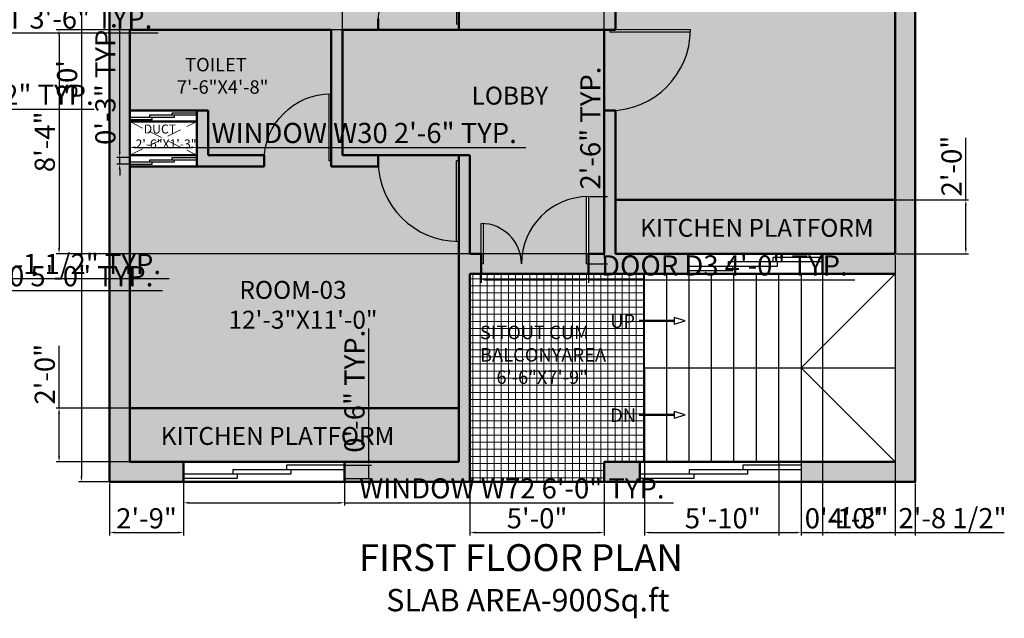
# Model space of a CAD drawing. Units: inches. Extents: x 3274 to 5176, y 1085 to 2172.
# Tile 9 of 16: x 3740 to 4180, y 1614 to 1881. Entities that reach past the tile are written whole.
import ezdxf

# ---------------------------------------------------------------- set-up
doc = ezdxf.new("R2010")
doc.units = ezdxf.units.IN
doc.linetypes.add('DASHED', pattern=[19.05, 12.7, -6.35])
for name, color, linetype, lineweight in [('A-ANNO-DIMS', 2, 'Continuous', 18), ('A-ANNO-TEXT', 7, 'Continuous', 25), ('A-AREA-IDEN', 3, 'Continuous', 25), ('A-DOOR', 4, 'Continuous', 25), ('A-FLOR-OPEN', 7, 'DASHED', 18), ('A-FLOR-PATT', 252, 'Continuous', 13), ('A-FLOR-STRS', 7, 'Continuous', 25), ('A-GLAZ', 5, 'Continuous', 25), ('A-WALL', 7, 'Continuous', 50), ('A-WALL-PATT', 8, 'Continuous', 13)]:
    doc.layers.add(name, color=color, linetype=linetype, lineweight=lineweight)
doc.styles.get("Standard").update_dxf_attribs({"font": 'arial.ttf'})
doc.dimstyles.new('ISO-25', dxfattribs={"dimtxt": 9, "dimasz": 2.5, "dimexe": 1.25, "dimexo": 0.625, "dimtad": 1, "dimdec": 1, "dimlunit": 3, "dimtxsty": 'Standard', "dimcen": 2.5, "dimclrd": 4, "dimclre": 4, "dimclrt": 1, "dimadec": 0, "dimazin": 0, "dimtfac": 1, "dimtdec": 1, "dimtmove": 0, "dimatfit": 3, "dimfxl": 1, "dimarcsym": 0})

# ---------------------------------------------------------------- blocks, each defined once
blk = doc.blocks.new('*D66')
at = {"layer": 'A-ANNO-DIMS', "color": 0, "lineweight": -2, "transparency": 16777216}
for p, q in [((3779.1, 2034.48), (3765.87, 2034.48)), ((3767.12, 2031.98), (3767.12, 1676.98)), ((3779.1, 1674.48), (3765.87, 1674.48))]:
    blk.add_line(p, q, dxfattribs=at)
at = {"layer": 'A-ANNO-DIMS', "color": 0, "transparency": 16777216}
for points in [[(3766.71, 2031.98), (3767.54, 2031.98), (3767.12, 2034.48)], [(3766.71, 1676.98), (3767.54, 1676.98), (3767.12, 1674.48)]]:
    blk.add_solid(points, dxfattribs=at)
at = {"layer": 'Defpoints', "color": 0, "transparency": 16777216}
for p in [(3779.73, 2034.48), (3767.12, 1674.48), (3779.73, 1674.48)]:
    blk.add_point(p, dxfattribs=at)
at = {"layer": 'A-ANNO-DIMS', "color": 0, "transparency": 16777216, "insert": (3761.9, 1854.48), "char_height": 9, "attachment_point": 5, "rotation": 90}
blk.add_mtext("30'", dxfattribs=at)
blk = doc.blocks.new('1')
for p, q in [((0, 36), (0, 0)), ((1, 36), (1, 0)), ((0, 0), (1, 0))]:
    blk.add_line(p, q)
blk.add_arc((0, 0), 36, 0, 90)
blk = doc.blocks.new('3')
for p, q in [((47, 30), (47, 0)), ((48, 30), (48, 0)), ((0, 0), (0, 18)), ((1, 0), (1, 18)), ((1, 0), (0, 0)), ((48, 0), (47, 0))]:
    blk.add_line(p, q)
for centre, radius, start, end in [((48, 0), 30, 90, 180), ((0, 0), 18, 0, 90)]:
    blk.add_arc(centre, radius, start, end)
blk = doc.blocks.new('2')
for p, q in [((0, 30), (0, 0)), ((1, 30), (1, 0)), ((0, 0), (1, 0))]:
    blk.add_line(p, q)
blk.add_arc((0, 0), 30, 0, 90)
blk = doc.blocks.new('WIN-30')
for p, q in [((4366.19, 1316.35), (4386.19, 1316.35)), ((4375.19, 1317.35), (4396.19, 1317.35)), ((4375.19, 1316.35), (4375.19, 1317.35)), ((4376.19, 1315.35), (4376.19, 1316.35)), ((4385.19, 1318.35), (4396.19, 1318.35)), ((4385.19, 1317.35), (4385.19, 1318.35)), ((4386.19, 1316.35), (4386.19, 1317.35)), ((4366.19, 1315.35), (4376.19, 1315.35))]:
    blk.add_line(p, q)
blk = doc.blocks.new('WIN-60')
for p, q in [((4598.19, 1271.85), (4640.19, 1271.85)), ((4598.19, 1269.85), (4598.19, 1271.85)), ((4618.19, 1273.85), (4640.19, 1273.85)), ((4618.19, 1271.85), (4618.19, 1273.85)), ((4620.19, 1269.85), (4620.19, 1271.85)), ((4580.19, 1269.85), (4620.19, 1269.85)), ((4580.19, 1267.85), (4600.19, 1267.85)), ((4600.19, 1267.85), (4600.19, 1269.85))]:
    blk.add_line(p, q)
blk = doc.blocks.new('WIN-72')
for p, q in [((4462.19, 1180.85), (4436.19, 1180.85)), ((4436.19, 1180.85), (4436.19, 1178.85)), ((4438.19, 1176.85), (4390.19, 1176.85)), ((4414.19, 1174.85), (4390.19, 1174.85)), ((4462.19, 1178.85), (4412.19, 1178.85)), ((4412.19, 1178.85), (4412.19, 1176.85)), ((4414.19, 1176.85), (4414.19, 1174.85)), ((4438.19, 1178.85), (4438.19, 1176.85))]:
    blk.add_line(p, q)
blk = doc.blocks.new('*D118')
at = {"layer": 'A-ANNO-DIMS', "color": 4, "lineweight": -2, "transparency": 16777216}
for p, q in [((3945.73, 1771.36), (3945.73, 1763.53)), ((3993.73, 1771.36), (3993.73, 1763.53)), ((3948.23, 1764.78), (3991.23, 1764.78)), ((3993.73, 1764.78), (4112.67, 1764.78))]:
    blk.add_line(p, q, dxfattribs=at)
at = {"layer": 'A-ANNO-DIMS', "color": 4, "transparency": 16777216}
for points in [[(3948.23, 1765.2), (3948.23, 1764.37), (3945.73, 1764.78)], [(3991.23, 1765.2), (3991.23, 1764.37), (3993.73, 1764.78)]]:
    blk.add_solid(points, dxfattribs=at)
at = {"layer": 'Defpoints', "color": 0, "transparency": 16777216}
for p in [(3945.73, 1771.98), (3993.73, 1771.98), (3993.73, 1764.78)]:
    blk.add_point(p, dxfattribs=at)
at = {"layer": 'A-ANNO-DIMS', "color": 1, "transparency": 16777216, "insert": (4054.45, 1770.07), "char_height": 9, "attachment_point": 5}
blk.add_mtext('DOOR D3 4\'-0" TYP.', dxfattribs=at)
blk = doc.blocks.new('*D119')
at = {"layer": 'A-ANNO-DIMS', "color": 4, "lineweight": -2, "transparency": 16777216}
for p, q in [((4000.93, 1801.98), (4000.93, 1860.75)), ((3994.35, 1801.98), (4002.18, 1801.98)), ((4000.93, 1774.48), (4000.93, 1799.48)), ((3994.35, 1771.98), (4002.18, 1771.98))]:
    blk.add_line(p, q, dxfattribs=at)
at = {"layer": 'A-ANNO-DIMS', "color": 4, "transparency": 16777216}
for points in [[(4000.51, 1799.48), (4001.35, 1799.48), (4000.93, 1801.98)], [(4000.51, 1774.48), (4001.35, 1774.48), (4000.93, 1771.98)]]:
    blk.add_solid(points, dxfattribs=at)
at = {"layer": 'Defpoints', "color": 0, "transparency": 16777216}
for p in [(3993.73, 1801.98), (4000.93, 1801.98), (3993.73, 1771.98)]:
    blk.add_point(p, dxfattribs=at)
at = {"layer": 'A-ANNO-DIMS', "color": 1, "transparency": 16777216, "insert": (3995.71, 1832.61), "char_height": 9, "attachment_point": 5, "rotation": 90}
blk.add_mtext('2\'-6" TYP.', dxfattribs=at)
blk = doc.blocks.new('*D120')
at = {"layer": 'A-ANNO-DIMS', "color": 4, "lineweight": -2, "transparency": 16777216}
for p, q in [((3788.73, 1820.11), (3788.73, 1825.23)), ((3791.23, 1823.98), (3816.23, 1823.98)), ((3818.73, 1820.11), (3818.73, 1825.23)), ((3818.73, 1823.98), (3965.71, 1823.98))]:
    blk.add_line(p, q, dxfattribs=at)
at = {"layer": 'A-ANNO-DIMS', "color": 4, "transparency": 16777216}
for points in [[(3791.23, 1824.4), (3791.23, 1823.57), (3788.73, 1823.98)], [(3816.23, 1824.4), (3816.23, 1823.57), (3818.73, 1823.98)]]:
    blk.add_solid(points, dxfattribs=at)
at = {"layer": 'Defpoints', "color": 0, "transparency": 16777216}
for p in [(3818.73, 1823.98), (3788.73, 1819.48), (3818.73, 1819.48)]:
    blk.add_point(p, dxfattribs=at)
at = {"layer": 'A-ANNO-DIMS', "color": 1, "transparency": 16777216, "insert": (3893.47, 1829.27), "char_height": 9, "attachment_point": 5}
blk.add_mtext('WINDOW W30 2\'-6" TYP.', dxfattribs=at)
blk = doc.blocks.new('*D121')
at = {"layer": 'A-ANNO-DIMS', "color": 4, "lineweight": -2, "transparency": 16777216}
for p, q in [((3784.23, 1821.98), (3784.23, 1880.59)), ((3788.1, 1819.48), (3782.98, 1819.48)), ((3784.23, 1816.48), (3784.23, 1819.48)), ((3788.1, 1816.48), (3782.98, 1816.48)), ((3784.23, 1813.98), (3784.23, 1811.48))]:
    blk.add_line(p, q, dxfattribs=at)
at = {"layer": 'A-ANNO-DIMS', "color": 4, "transparency": 16777216}
for points in [[(3783.81, 1821.98), (3784.65, 1821.98), (3784.23, 1819.48)], [(3783.81, 1813.98), (3784.65, 1813.98), (3784.23, 1816.48)]]:
    blk.add_solid(points, dxfattribs=at)
at = {"layer": 'Defpoints', "color": 0, "transparency": 16777216}
for p in [(3784.23, 1819.48), (3788.73, 1819.48), (3788.73, 1816.48)]:
    blk.add_point(p, dxfattribs=at)
at = {"layer": 'A-ANNO-DIMS', "color": 1, "transparency": 16777216, "insert": (3779.01, 1852.54), "char_height": 9, "attachment_point": 5, "rotation": 90}
blk.add_mtext('0\'-3" TYP.', dxfattribs=at)
blk = doc.blocks.new('*D124')
at = {"layer": 'A-ANNO-DIMS', "color": 4, "lineweight": -2, "transparency": 16777216}
for p, q in [((3812.73, 1675.36), (3812.73, 1663.93)), ((3884.73, 1675.36), (3884.73, 1663.93)), ((3815.23, 1665.18), (3882.23, 1665.18)), ((3884.73, 1665.18), (4031.71, 1665.18))]:
    blk.add_line(p, q, dxfattribs=at)
at = {"layer": 'A-ANNO-DIMS', "color": 4, "transparency": 16777216}
for points in [[(3815.23, 1665.6), (3815.23, 1664.77), (3812.73, 1665.18)], [(3882.23, 1665.6), (3882.23, 1664.77), (3884.73, 1665.18)]]:
    blk.add_solid(points, dxfattribs=at)
at = {"layer": 'Defpoints', "color": 0, "transparency": 16777216}
for p in [(3812.73, 1675.98), (3884.73, 1675.98), (3884.73, 1665.18)]:
    blk.add_point(p, dxfattribs=at)
at = {"layer": 'A-ANNO-DIMS', "color": 1, "transparency": 16777216, "insert": (3959.47, 1670.46), "char_height": 9, "attachment_point": 5}
blk.add_mtext('WINDOW W72 6\'-0" TYP.', dxfattribs=at)
blk = doc.blocks.new('*D125')
at = {"layer": 'A-ANNO-DIMS', "color": 4, "lineweight": -2, "transparency": 16777216}
for p, q in [((3895.53, 1684.48), (3895.53, 1743.09)), ((3885.35, 1681.98), (3896.78, 1681.98)), ((3895.53, 1675.98), (3895.53, 1681.98)), ((3885.35, 1675.98), (3896.78, 1675.98)), ((3895.53, 1673.48), (3895.53, 1670.98))]:
    blk.add_line(p, q, dxfattribs=at)
at = {"layer": 'A-ANNO-DIMS', "color": 4, "transparency": 16777216}
for points in [[(3895.11, 1684.48), (3895.95, 1684.48), (3895.53, 1681.98)], [(3895.11, 1673.48), (3895.95, 1673.48), (3895.53, 1675.98)]]:
    blk.add_solid(points, dxfattribs=at)
at = {"layer": 'Defpoints', "color": 0, "transparency": 16777216}
for p in [(3884.73, 1681.98), (3895.53, 1681.98), (3884.73, 1675.98)]:
    blk.add_point(p, dxfattribs=at)
at = {"layer": 'A-ANNO-DIMS', "color": 1, "transparency": 16777216, "insert": (3890.31, 1715.04), "char_height": 9, "attachment_point": 5, "rotation": 90}
blk.add_mtext('0\'-6" TYP.', dxfattribs=at)
blk = doc.blocks.new('*D128')
at = {"layer": 'A-ANNO-DIMS', "color": 4, "lineweight": -2, "transparency": 16777216}
for p, q in [((3596.3, 1768.36), (3596.3, 1758.73)), ((3656.3, 1768.36), (3656.3, 1758.73)), ((3598.8, 1759.98), (3653.8, 1759.98)), ((3656.3, 1759.98), (3803.28, 1759.98))]:
    blk.add_line(p, q, dxfattribs=at)
at = {"layer": 'A-ANNO-DIMS', "color": 4, "transparency": 16777216}
for points in [[(3598.8, 1760.4), (3598.8, 1759.57), (3596.3, 1759.98)], [(3653.8, 1760.4), (3653.8, 1759.57), (3656.3, 1759.98)]]:
    blk.add_solid(points, dxfattribs=at)
at = {"layer": 'Defpoints', "color": 0, "transparency": 16777216}
for p in [(3596.3, 1768.98), (3656.3, 1768.98), (3656.3, 1759.98)]:
    blk.add_point(p, dxfattribs=at)
at = {"layer": 'A-ANNO-DIMS', "color": 1, "transparency": 16777216, "insert": (3731.04, 1765.26), "char_height": 9, "attachment_point": 5}
blk.add_mtext('WINDOW W60 5\'-0" TYP.', dxfattribs=at)
blk = doc.blocks.new('*D130')
at = {"layer": 'A-ANNO-DIMS', "color": 4, "lineweight": -2, "transparency": 16777216}
for p, q in [((3648.04, 1880.86), (3648.04, 1873.91)), ((3690.17, 1880.86), (3690.17, 1873.91)), ((3650.54, 1875.16), (3687.67, 1875.16)), ((3690.17, 1875.16), (3801.39, 1875.16))]:
    blk.add_line(p, q, dxfattribs=at)
at = {"layer": 'A-ANNO-DIMS', "color": 4, "transparency": 16777216}
for points in [[(3650.54, 1875.58), (3650.54, 1874.75), (3648.04, 1875.16)], [(3687.67, 1875.58), (3687.67, 1874.75), (3690.17, 1875.16)]]:
    blk.add_solid(points, dxfattribs=at)
at = {"layer": 'Defpoints', "color": 0, "transparency": 16777216}
for p in [(3648.04, 1881.48), (3690.17, 1881.48), (3690.17, 1875.16)]:
    blk.add_point(p, dxfattribs=at)
at = {"layer": 'A-ANNO-DIMS', "color": 1, "transparency": 16777216, "insert": (3747.03, 1880.39), "char_height": 9, "attachment_point": 5}
blk.add_mtext('TV UNIT 3\'-6" TYP.', dxfattribs=at)
blk = doc.blocks.new('*D139')
at = {"layer": 'A-ANNO-DIMS', "color": 4, "lineweight": -2, "transparency": 16777216}
for p, q in [((3664.71, 1838.01), (3664.71, 1842.31)), ((3667.21, 1841.06), (3684.52, 1841.06)), ((3687.02, 1838.01), (3687.02, 1842.31)), ((3687.02, 1841.06), (3772.75, 1841.06))]:
    blk.add_line(p, q, dxfattribs=at)
at = {"layer": 'A-ANNO-DIMS', "color": 4, "transparency": 16777216}
for points in [[(3667.21, 1841.48), (3667.21, 1840.65), (3664.71, 1841.06)], [(3684.52, 1841.48), (3684.52, 1840.65), (3687.02, 1841.06)]]:
    blk.add_solid(points, dxfattribs=at)
at = {"layer": 'Defpoints', "color": 0, "transparency": 16777216}
for p in [(3687.02, 1841.06), (3664.71, 1837.38), (3687.02, 1837.38)]:
    blk.add_point(p, dxfattribs=at)
at = {"layer": 'A-ANNO-DIMS', "color": 1, "transparency": 16777216, "insert": (3731.13, 1846.34), "char_height": 9, "attachment_point": 5}
blk.add_mtext('1\'-10 1/2" TYP.', dxfattribs=at)
blk = doc.blocks.new('*D140')
at = {"layer": 'A-ANNO-DIMS', "color": 4, "lineweight": -2, "transparency": 16777216}
for p, q in [((3596.75, 1775.85), (3596.75, 1764.21)), ((3670.16, 1775.85), (3670.16, 1764.21)), ((3599.25, 1765.46), (3667.66, 1765.46)), ((3670.16, 1765.46), (3806.3, 1765.46))]:
    blk.add_line(p, q, dxfattribs=at)
at = {"layer": 'A-ANNO-DIMS', "color": 4, "transparency": 16777216}
for points in [[(3599.25, 1765.88), (3599.25, 1765.04), (3596.75, 1765.46)], [(3667.66, 1765.88), (3667.66, 1765.04), (3670.16, 1765.46)]]:
    blk.add_solid(points, dxfattribs=at)
at = {"layer": 'Defpoints', "color": 0, "transparency": 16777216}
for p in [(3596.75, 1776.47), (3670.16, 1776.47), (3670.16, 1765.46)]:
    blk.add_point(p, dxfattribs=at)
at = {"layer": 'A-ANNO-DIMS', "color": 1, "transparency": 16777216, "insert": (3739.48, 1770.74), "char_height": 9, "attachment_point": 5}
blk.add_mtext('SOFA S1 6\'-1 1/2" TYP.', dxfattribs=at)
blk = doc.blocks.new('*D204')
at = {"layer": 'A-ANNO-DIMS', "color": 4, "lineweight": -2, "transparency": 16777216}
for p, q in [((3779.73, 1673.86), (3779.73, 1650.63)), ((3812.73, 1673.86), (3812.73, 1650.63)), ((3782.23, 1651.88), (3810.23, 1651.88))]:
    blk.add_line(p, q, dxfattribs=at)
at = {"layer": 'A-ANNO-DIMS', "color": 4, "transparency": 16777216}
for points in [[(3782.23, 1652.3), (3782.23, 1651.47), (3779.73, 1651.88)], [(3810.23, 1652.3), (3810.23, 1651.47), (3812.73, 1651.88)]]:
    blk.add_solid(points, dxfattribs=at)
at = {"layer": 'Defpoints', "color": 0, "transparency": 16777216}
for p in [(3779.73, 1674.48), (3812.73, 1674.48), (3812.73, 1651.88)]:
    blk.add_point(p, dxfattribs=at)
at = {"layer": 'A-ANNO-DIMS', "color": 1, "transparency": 16777216, "insert": (3796.23, 1657.1), "char_height": 9, "attachment_point": 5}
blk.add_mtext('2\'-9"', dxfattribs=at)
blk = doc.blocks.new('*D205')
at = {"layer": 'A-ANNO-DIMS', "color": 4, "lineweight": -2, "transparency": 16777216}
for p, q in [((4088.73, 1673.86), (4088.73, 1650.63)), ((4139.73, 1673.86), (4139.73, 1650.63)), ((4091.23, 1651.88), (4137.23, 1651.88))]:
    blk.add_line(p, q, dxfattribs=at)
at = {"layer": 'A-ANNO-DIMS', "color": 4, "transparency": 16777216}
for points in [[(4091.23, 1652.3), (4091.23, 1651.47), (4088.73, 1651.88)], [(4137.23, 1652.3), (4137.23, 1651.47), (4139.73, 1651.88)]]:
    blk.add_solid(points, dxfattribs=at)
at = {"layer": 'Defpoints', "color": 0, "transparency": 16777216}
for p in [(4088.73, 1674.48), (4139.73, 1674.48), (4139.73, 1651.88)]:
    blk.add_point(p, dxfattribs=at)
at = {"layer": 'A-ANNO-DIMS', "color": 1, "transparency": 16777216, "insert": (4114.23, 1657.11), "char_height": 9, "attachment_point": 5}
blk.add_mtext('4\'-3"', dxfattribs=at)
blk = doc.blocks.new('*D206')
at = {"layer": 'A-ANNO-DIMS', "color": 4, "lineweight": -2, "transparency": 16777216}
for p, q in [((3940.73, 1673.86), (3940.73, 1650.63)), ((4000.73, 1673.86), (4000.73, 1650.63)), ((3943.23, 1651.88), (3998.23, 1651.88))]:
    blk.add_line(p, q, dxfattribs=at)
at = {"layer": 'A-ANNO-DIMS', "color": 4, "transparency": 16777216}
for points in [[(3943.23, 1652.3), (3943.23, 1651.47), (3940.73, 1651.88)], [(3998.23, 1652.3), (3998.23, 1651.47), (4000.73, 1651.88)]]:
    blk.add_solid(points, dxfattribs=at)
at = {"layer": 'Defpoints', "color": 0, "transparency": 16777216}
for p in [(3940.73, 1674.48), (4000.73, 1674.48), (4000.73, 1651.88)]:
    blk.add_point(p, dxfattribs=at)
at = {"layer": 'A-ANNO-DIMS', "color": 1, "transparency": 16777216, "insert": (3970.73, 1657.1), "char_height": 9, "attachment_point": 5}
blk.add_mtext('5\'-0"', dxfattribs=at)
blk = doc.blocks.new('*D207')
at = {"layer": 'A-ANNO-DIMS', "color": 4, "lineweight": -2, "transparency": 16777216}
for p, q in [((3757.13, 1707.48), (3757.13, 1735.31)), ((3935.1, 1707.48), (3755.88, 1707.48)), ((3757.13, 1685.98), (3757.13, 1704.98)), ((3935.1, 1683.48), (3755.88, 1683.48))]:
    blk.add_line(p, q, dxfattribs=at)
at = {"layer": 'A-ANNO-DIMS', "color": 4, "transparency": 16777216}
for points in [[(3756.71, 1704.98), (3757.55, 1704.98), (3757.13, 1707.48)], [(3756.71, 1685.98), (3757.55, 1685.98), (3757.13, 1683.48)]]:
    blk.add_solid(points, dxfattribs=at)
at = {"layer": 'Defpoints', "color": 0, "transparency": 16777216}
for p in [(3757.13, 1707.48), (3935.73, 1707.48), (3935.73, 1683.48)]:
    blk.add_point(p, dxfattribs=at)
at = {"layer": 'A-ANNO-DIMS', "color": 1, "transparency": 16777216, "insert": (3751.91, 1722.65), "char_height": 9, "attachment_point": 5, "rotation": 90}
blk.add_mtext('2\'-0"', dxfattribs=at)
blk = doc.blocks.new('*D209')
at = {"layer": 'A-ANNO-DIMS', "color": 4, "lineweight": -2, "transparency": 16777216}
for p, q in [((4162.33, 1800.48), (4162.33, 1828.31)), ((4131.35, 1800.48), (4163.58, 1800.48)), ((4162.33, 1778.98), (4162.33, 1797.98)), ((4131.35, 1776.48), (4163.58, 1776.48))]:
    blk.add_line(p, q, dxfattribs=at)
at = {"layer": 'A-ANNO-DIMS', "color": 4, "transparency": 16777216}
for points in [[(4161.91, 1797.98), (4162.75, 1797.98), (4162.33, 1800.48)], [(4161.91, 1778.98), (4162.75, 1778.98), (4162.33, 1776.48)]]:
    blk.add_solid(points, dxfattribs=at)
at = {"layer": 'Defpoints', "color": 0, "transparency": 16777216}
for p in [(4130.73, 1800.48), (4162.33, 1800.48), (4130.73, 1776.48)]:
    blk.add_point(p, dxfattribs=at)
at = {"layer": 'A-ANNO-DIMS', "color": 1, "transparency": 16777216, "insert": (4157.11, 1815.65), "char_height": 9, "attachment_point": 5, "rotation": 90}
blk.add_mtext('2\'-0"', dxfattribs=at)
blk = doc.blocks.new('*D210')
at = {"layer": 'A-ANNO-DIMS', "color": 4, "lineweight": -2, "transparency": 16777216}
for p, q in [((4018.73, 1724.86), (4018.73, 1650.63)), ((4088.73, 1724.86), (4088.73, 1650.63)), ((4021.23, 1651.88), (4086.23, 1651.88))]:
    blk.add_line(p, q, dxfattribs=at)
at = {"layer": 'A-ANNO-DIMS', "color": 4, "transparency": 16777216}
for points in [[(4021.23, 1652.3), (4021.23, 1651.47), (4018.73, 1651.88)], [(4086.23, 1652.3), (4086.23, 1651.47), (4088.73, 1651.88)]]:
    blk.add_solid(points, dxfattribs=at)
at = {"layer": 'Defpoints', "color": 0, "transparency": 16777216}
for p in [(4018.73, 1725.48), (4088.73, 1725.48), (4088.73, 1651.88)]:
    blk.add_point(p, dxfattribs=at)
at = {"layer": 'A-ANNO-DIMS', "color": 1, "transparency": 16777216, "insert": (4053.73, 1657.1), "char_height": 9, "attachment_point": 5}
blk.add_mtext('5\'-10"', dxfattribs=at)
blk = doc.blocks.new('*D211')
at = {"layer": 'A-ANNO-DIMS', "color": 4, "lineweight": -2, "transparency": 16777216}
for p, q in [((4078.73, 1682.86), (4078.73, 1650.63)), ((4088.73, 1682.86), (4088.73, 1650.63)), ((4081.23, 1651.88), (4086.23, 1651.88)), ((4088.73, 1651.88), (4123.4, 1651.88))]:
    blk.add_line(p, q, dxfattribs=at)
at = {"layer": 'A-ANNO-DIMS', "color": 4, "transparency": 16777216}
for points in [[(4081.23, 1652.3), (4081.23, 1651.47), (4078.73, 1651.88)], [(4086.23, 1652.3), (4086.23, 1651.47), (4088.73, 1651.88)]]:
    blk.add_solid(points, dxfattribs=at)
at = {"layer": 'Defpoints', "color": 0, "transparency": 16777216}
for p in [(4078.73, 1683.48), (4088.73, 1683.48), (4088.73, 1651.88)]:
    blk.add_point(p, dxfattribs=at)
at = {"layer": 'A-ANNO-DIMS', "color": 1, "transparency": 16777216, "insert": (4107.31, 1657.1), "char_height": 9, "attachment_point": 5}
blk.add_mtext('0\'-10"', dxfattribs=at)
blk = doc.blocks.new('*D212')
at = {"layer": 'A-ANNO-DIMS', "color": 4, "lineweight": -2, "transparency": 16777216}
for p, q in [((3883.73, 1877.11), (3883.73, 2058.33)), ((3886.23, 2057.08), (3998.23, 2057.08)), ((4000.73, 1841.11), (4000.73, 2058.33))]:
    blk.add_line(p, q, dxfattribs=at)
at = {"layer": 'A-ANNO-DIMS', "color": 4, "transparency": 16777216}
for points in [[(3886.23, 2057.5), (3886.23, 2056.67), (3883.73, 2057.08)], [(3998.23, 2057.5), (3998.23, 2056.67), (4000.73, 2057.08)]]:
    blk.add_solid(points, dxfattribs=at)
at = {"layer": 'Defpoints', "color": 0, "transparency": 16777216}
for p in [(4000.73, 2057.08), (3883.73, 1876.48), (4000.73, 1840.48)]:
    blk.add_point(p, dxfattribs=at)
at = {"layer": 'A-ANNO-DIMS', "color": 1, "transparency": 16777216, "insert": (3942.23, 2062.3), "char_height": 9, "attachment_point": 5}
blk.add_mtext('9\'-9"', dxfattribs=at)
blk = doc.blocks.new('*D213')
at = {"layer": 'A-ANNO-DIMS', "color": 4, "lineweight": -2, "transparency": 16777216}
for p, q in [((3935.1, 1876.48), (3755.88, 1876.48)), ((3757.13, 1873.98), (3757.13, 1778.98)), ((4000.1, 1776.48), (3755.88, 1776.48))]:
    blk.add_line(p, q, dxfattribs=at)
at = {"layer": 'A-ANNO-DIMS', "color": 4, "transparency": 16777216}
for points in [[(3756.71, 1873.98), (3757.55, 1873.98), (3757.13, 1876.48)], [(3756.71, 1778.98), (3757.55, 1778.98), (3757.13, 1776.48)]]:
    blk.add_solid(points, dxfattribs=at)
at = {"layer": 'Defpoints', "color": 0, "transparency": 16777216}
for p in [(3935.73, 1876.48), (3757.13, 1776.48), (4000.73, 1776.48)]:
    blk.add_point(p, dxfattribs=at)
at = {"layer": 'A-ANNO-DIMS', "color": 1, "transparency": 16777216, "insert": (3751.91, 1826.48), "char_height": 9, "attachment_point": 5, "rotation": 90}
blk.add_mtext('8\'-4"', dxfattribs=at)
blk = doc.blocks.new('*D214')
at = {"layer": 'A-ANNO-DIMS', "color": 4, "lineweight": -2, "transparency": 16777216}
for p, q in [((4098.23, 1775.86), (4098.23, 1650.63)), ((4130.73, 1775.86), (4130.73, 1650.63)), ((4100.73, 1651.88), (4128.23, 1651.88)), ((4130.73, 1651.88), (4179.53, 1651.88))]:
    blk.add_line(p, q, dxfattribs=at)
at = {"layer": 'A-ANNO-DIMS', "color": 4, "transparency": 16777216}
for points in [[(4100.73, 1652.3), (4100.73, 1651.47), (4098.23, 1651.88)], [(4128.23, 1652.3), (4128.23, 1651.47), (4130.73, 1651.88)]]:
    blk.add_solid(points, dxfattribs=at)
at = {"layer": 'Defpoints', "color": 0, "transparency": 16777216}
for p in [(4098.23, 1776.48), (4130.73, 1776.48), (4130.73, 1651.88)]:
    blk.add_point(p, dxfattribs=at)
at = {"layer": 'A-ANNO-DIMS', "color": 1, "transparency": 16777216, "insert": (4156.38, 1657.16), "char_height": 9, "attachment_point": 5}
blk.add_mtext('2\'-8 1/2"', dxfattribs=at)

msp = doc.modelspace()

# ---------------------------------------------------------------- hatches: boundary and pattern name
at = {"layer": 'A-FLOR-PATT'}
h = msp.add_hatch(color=256, dxfattribs=at)
h.dxf.hatch_style = 1
h.paths.add_polyline_path([(4130.73, 2007.48), (4094.73, 2007.48), (4094.73, 1995.48), (4092.23, 1995.48, 0.404482), (4062.25, 1966.48), (4092.23, 1966.48), (4092.23, 1965.48), (4094.73, 1965.48), (4094.73, 1960.48), (4005.73, 1960.48), (4005.73, 1876.48), (4039.23, 1876.48, -0.394001), (4005.73, 1840.57), (4005.73, 1800.48), (4130.73, 1800.48)])
h.paths.add_polyline_path([(4089.73, 1995.38), (4089.73, 2025.48), (4005.73, 2025.48), (4005.73, 1965.48), (4062.23, 1965.48, -0.389983)])
h.paths.add_polyline_path([(4039.22, 1875.48), (4003.23, 1875.48), (4003.23, 1876.48), (4000.73, 1876.48), (4000.73, 1840.48), (4003.23, 1840.48, 0.4061)])
h.paths.add_polyline_path([(4043.84, 1879.07), (4112.24, 1879.07), (4112.24, 1908.93), (4043.84, 1908.93)], flags=24)
h.paths.add_polyline_path([(4026.66, 1988.49), (4068.63, 1988.49), (4068.63, 2010.88), (4026.66, 2010.88)], flags=24)
h = msp.add_hatch(color=256, dxfattribs=at)
h.dxf.hatch_style = 1
h.paths.add_polyline_path([(3938.23, 1949.48), (3935.73, 1949.48), (3935.73, 2001.48), (3788.73, 2001.48), (3788.73, 1881.48), (3899.82, 1881.48, -0.394001), (3935.73, 1914.98), (3935.73, 1919.48), (3938.23, 1919.48), (3938.23, 1920.48), (3968.21, 1920.48, 0.404482)])
h.paths.add_polyline_path([(3934.73, 1914.97, 0.4061), (3899.73, 1878.98), (3899.73, 1876.48), (3935.73, 1876.48), (3935.73, 1878.98), (3934.73, 1878.98)])
h.paths.add_polyline_path([(4000.73, 1984.48), (3940.73, 1984.48), (3940.73, 1949.38, -0.389983), (3968.23, 1919.48), (3940.73, 1919.48), (3940.73, 1881.48), (4000.73, 1881.48)])
h.paths.add_polyline_path([(3829.62, 1944.89), (3898.01, 1944.89), (3898.01, 1974.74), (3829.62, 1974.74)], flags=24)
h.paths.add_polyline_path([(3951.89, 1951.36), (3993.86, 1951.36), (3993.86, 1973.74), (3951.89, 1973.74)], flags=24)
h = msp.add_hatch(color=256, dxfattribs=at)
h.dxf.hatch_style = 1
h.paths.add_polyline_path([(3899.82, 1815.48), (3878.73, 1815.48), (3878.73, 1817.98), (3877.73, 1817.98), (3877.73, 1847.97, 0.404482), (3848.73, 1817.98), (3848.73, 1815.48), (3788.73, 1815.48), (3788.73, 1707.48), (3935.73, 1707.48), (3935.73, 1781.98, -0.394001)])
h.paths.add_polyline_path([(3878.73, 1847.98), (3878.73, 1876.48), (3788.73, 1876.48), (3788.73, 1840.48), (3823.73, 1840.48), (3823.73, 1820.48), (3848.83, 1820.48, -0.389983)])
h.paths.add_polyline_path([(3934.73, 1817.98), (3935.73, 1817.98), (3935.73, 1820.48), (3899.73, 1820.48), (3899.73, 1817.98, 0.4061), (3934.73, 1782)], flags=17)
h.paths.add_polyline_path([(3829.62, 1738.43), (3898.01, 1738.43), (3898.01, 1768.28), (3829.62, 1768.28)], flags=24)
h.paths.add_polyline_path([(3807.9, 1844.56), (3849.87, 1844.56), (3849.87, 1866.94), (3807.9, 1866.94)], flags=24)
h = msp.add_hatch(color=256, dxfattribs=at)
h.dxf.hatch_style = 1
h.paths.add_polyline_path([(3899.73, 1876.48), (3883.73, 1876.48), (3883.73, 1820.48), (3899.73, 1820.48), (3935.73, 1820.48), (3940.73, 1820.48), (3940.73, 1776.48), (3945.73, 1776.48), (3945.73, 1789.98, -0.414214), (3963.73, 1771.98, -0.404482), (3992.73, 1801.97), (3992.73, 1801.98), (3993.73, 1801.98), (3993.73, 1776.48), (4000.73, 1776.48), (4000.73, 1840.48), (4000.73, 1876.48), (3935.73, 1876.48)])
h.paths.add_polyline_path([(3963.73, 1771.98, 0.398025), (3946.73, 1789.96), (3946.73, 1771.98), (3945.73, 1767.48), (3993.73, 1767.48), (3993.73, 1771.98), (3992.73, 1771.98), (3992.73, 1801.97, 0.404482)])
h.paths.add_polyline_path([(3938.66, 1838.59), (3979.93, 1838.59), (3979.93, 1855.08), (3938.66, 1855.08)], flags=24)
h = msp.add_hatch(color=256, dxfattribs=at)
h.dxf.hatch_style = 1
h.paths.add_polyline_path([(4005.73, 1776.48), (4130.73, 1776.48), (4130.73, 1800.48), (4005.73, 1800.48)])
h.paths.add_polyline_path([(4013.96, 1779.54), (4130.97, 1779.54), (4130.97, 1796.03), (4013.96, 1796.03)], flags=9)
h = msp.add_hatch(dxfattribs=at)
h.set_pattern_fill('ANSI37', color=256, angle=45)
h.set_pattern_definition([(90, (-433.0866, 0), (-3.175, 0), []), (180, (-433.0866, 0), (-2e-16, -3.175), [])])
h.paths.add_polyline_path([(3940.73, 1674.48), (4000.73, 1674.48), (4000.73, 1683.48), (4018.73, 1683.48), (4018.73, 1725.48), (4018.73, 1767.48), (3993.73, 1767.48), (3945.73, 1767.48), (3940.73, 1767.48)])
h.paths.add_polyline_path([(3943.12, 1714.79), (4009.02, 1714.79), (4009.02, 1747.29), (3943.12, 1747.29)], flags=24)
h.paths.add_polyline_path([(4001.92, 1741.7), (4016.61, 1741.7), (4016.61, 1750.85), (4001.92, 1750.85)], flags=24)
h.paths.add_polyline_path([(4001.94, 1699.83), (4017.05, 1699.83), (4017.05, 1708.83), (4001.94, 1708.83)], flags=24)
h = msp.add_hatch(color=256, dxfattribs=at)
h.dxf.hatch_style = 1
h.paths.add_polyline_path([(3788.73, 1707.48), (3788.73, 1683.48), (3935.73, 1683.48), (3935.73, 1707.48)])
h.paths.add_polyline_path([(3799.76, 1686.54), (3916.77, 1686.54), (3916.77, 1703.03), (3799.76, 1703.03)], flags=24)
at = {"layer": 'A-WALL-PATT'}
h = msp.add_hatch(color=256, dxfattribs=at)
h.dxf.hatch_style = 1
h.paths.add_polyline_path([(3848.73, 1820.48), (3823.73, 1820.48), (3823.73, 1840.48), (3818.73, 1840.48), (3818.73, 1815.48), (3848.73, 1815.48)], flags=17)
h.paths.add_polyline_path([(3788.73, 1876.48), (3878.73, 1876.48), (3878.73, 1815.48), (3899.73, 1815.48), (3899.73, 1820.48), (3883.73, 1820.48), (3883.73, 1876.48), (3899.73, 1876.48), (3899.73, 1881.48), (3788.73, 1881.48), (3788.73, 2025.48), (4089.73, 2025.48), (4089.73, 1995.48), (4094.73, 1995.48), (4094.73, 2025.48), (4130.73, 2025.48), (4130.73, 1776.48), (4098.23, 1776.48), (4098.23, 1767.48), (4130.73, 1767.48), (4130.73, 1683.48), (4088.73, 1683.48), (4088.73, 1674.48), (4139.73, 1674.48), (4139.73, 2034.48), (3779.73, 2034.48), (3779.73, 1674.48), (3812.73, 1674.48), (3812.73, 1683.48), (3788.73, 1683.48)])
h.paths.add_polyline_path([(4005.73, 1989.48), (3982.73, 1989.48), (3982.73, 1984.48), (4000.73, 1984.48), (4000.73, 1881.48), (3940.73, 1881.48), (3940.73, 1919.48), (3938.23, 1919.48), (3935.73, 1919.48), (3935.73, 1876.48), (4005.73, 1876.48), (4005.73, 1960.48), (4094.73, 1960.48), (4094.73, 1965.48), (4005.73, 1965.48)], flags=17)
h.paths.add_polyline_path([(3958.73, 1989.48), (3935.73, 1989.48), (3935.73, 1949.48), (3940.73, 1949.48), (3940.73, 1984.48), (3958.73, 1984.48)], flags=17)
h.paths.add_polyline_path([(4038.23, 1776.48), (4005.73, 1776.48), (4005.73, 1840.48), (4000.73, 1840.48), (4000.73, 1776.48), (3993.73, 1776.48), (3993.73, 1771.98), (3993.73, 1767.48), (4038.23, 1767.48)], flags=17)
h.paths.add_polyline_path([(3940.73, 1767.48), (3945.73, 1767.48), (3945.73, 1776.48), (3940.73, 1776.48), (3940.73, 1820.48), (3935.73, 1820.48), (3935.73, 1683.48), (3884.73, 1683.48), (3884.73, 1674.48), (3940.73, 1674.48)], flags=17)
h.paths.add_polyline_path([(4016.73, 1683.48), (4000.73, 1683.48), (4000.73, 1674.48), (4016.73, 1674.48)], flags=17)

# ---------------------------------------------------------------- linework, layer by layer
at = {"layer": 'A-FLOR-OPEN', "ltscale": 0.5}
for p, q in [((3788.73, 1835.48), (3818.73, 1820.48)), ((3788.73, 1820.48), (3818.73, 1835.48))]:
    msp.add_line(p, q, dxfattribs=at)
at = {"layer": 'A-FLOR-STRS'}
for p, q in [((4018.73, 1725.48), (4018.73, 1767.48)), ((4028.73, 1725.48), (4028.73, 1767.48)), ((4038.73, 1725.48), (4038.73, 1767.48)), ((4048.73, 1725.48), (4048.73, 1767.48)), ((4058.73, 1725.48), (4058.73, 1767.48)), ((4068.73, 1725.48), (4068.73, 1767.48)), ((4078.73, 1725.48), (4078.73, 1767.48)), ((4088.73, 1767.48), (4088.73, 1683.48)), ((4088.73, 1725.48), (4130.73, 1767.48)), ((4130.73, 1767.48), (4130.73, 1683.48)), ((4018.73, 1725.48), (4130.73, 1725.48)), ((4018.73, 1683.48), (4018.73, 1725.48)), ((4028.73, 1683.48), (4028.73, 1725.48)), ((4038.73, 1683.48), (4038.73, 1725.48)), ((4048.73, 1683.48), (4048.73, 1725.48)), ((4058.73, 1683.48), (4058.73, 1725.48)), ((4068.73, 1683.48), (4068.73, 1725.48)), ((4078.73, 1683.48), (4078.73, 1725.48)), ((4088.73, 1725.48), (4130.73, 1683.48)), ((4088.73, 1683.48), (4088.73, 1674.48))]:
    msp.add_line(p, q, dxfattribs=at)
for points in [[(4036.93, 1746.48), (4032.04, 1747.98), (4032.04, 1744.98)], [(4036.93, 1704.48), (4032.04, 1705.98), (4032.04, 1702.98)]]:
    msp.add_lwpolyline(points, close=True, dxfattribs=at)
at = {"layer": 'A-WALL'}
for p, q in [((4130.73, 2025.48), (4130.73, 1776.48)), ((4005.73, 1960.48), (4005.73, 1876.48)), ((3935.73, 1876.48), (3935.73, 1919.48)), ((3899.73, 1876.48), (3899.73, 1881.48)), ((3788.73, 1876.48), (3878.73, 1876.48)), ((3788.73, 1683.48), (3788.73, 1876.48)), ((3878.73, 1815.48), (3878.73, 1876.48)), ((3883.73, 1876.48), (3899.73, 1876.48)), ((3883.73, 1820.48), (3883.73, 1876.48)), ((3899.73, 1876.48), (3935.73, 1876.48)), ((3935.73, 1876.48), (4005.73, 1876.48)), ((4000.73, 1840.48), (4000.73, 1876.48)), ((3788.73, 1840.48), (3823.73, 1840.48)), ((3818.73, 1815.48), (3818.73, 1840.48)), ((3823.73, 1820.48), (3823.73, 1840.48)), ((4000.73, 1840.48), (4005.73, 1840.48)), ((4000.73, 1840.48), (4000.73, 1776.48)), ((4005.73, 1840.48), (4005.73, 1776.48)), ((3788.73, 1835.48), (3818.73, 1835.48)), ((3788.73, 1820.48), (3818.73, 1820.48)), ((3823.73, 1820.48), (3848.73, 1820.48)), ((3848.73, 1815.48), (3848.73, 1820.48)), ((3883.73, 1820.48), (3899.73, 1820.48)), ((3899.73, 1815.48), (3899.73, 1820.48)), ((3935.73, 1820.48), (3899.73, 1820.48)), ((3935.73, 1820.48), (3940.73, 1820.48)), ((3935.73, 1683.48), (3935.73, 1820.48)), ((3940.73, 1776.48), (3940.73, 1820.48)), ((3788.73, 1815.48), (3848.73, 1815.48)), ((3878.73, 1815.48), (3899.73, 1815.48)), ((4005.73, 1800.48), (4130.73, 1800.48)), ((3940.73, 1776.48), (3945.73, 1776.48)), ((3945.73, 1767.48), (3945.73, 1776.48)), ((3993.73, 1776.48), (4000.73, 1776.48)), ((3993.73, 1767.48), (3993.73, 1776.48)), ((4005.73, 1776.48), (4130.73, 1776.48)), ((4038.23, 1767.48), (4038.23, 1776.48)), ((4098.23, 1767.48), (4098.23, 1776.48)), ((3940.73, 1767.48), (3945.73, 1767.48)), ((3940.73, 1674.48), (3940.73, 1767.48)), ((3993.73, 1767.48), (3945.73, 1767.48)), ((3993.73, 1767.48), (4130.73, 1767.48)), ((4016.29, 1746.48), (4032.04, 1746.48)), ((3935.73, 1707.48), (3788.73, 1707.48)), ((4016.29, 1704.48), (4032.04, 1704.48)), ((3935.73, 1683.48), (3788.73, 1683.48)), ((3812.73, 1683.48), (3812.73, 1674.48)), ((3884.73, 1683.48), (3884.73, 1674.48)), ((4130.73, 1683.48), (4000.73, 1683.48)), ((4000.73, 1674.48), (4000.73, 1683.48)), ((4016.73, 1683.48), (4016.73, 1674.48))]:
    msp.add_line(p, q, dxfattribs=at)
msp.add_lwpolyline([(3940.73, 1674.48), (3779.73, 1674.48), (3779.73, 2034.48), (4139.73, 2034.48), (4139.73, 1674.48), (3940.73, 1674.48)], dxfattribs=at)

# ---------------------------------------------------------------- block references
at = {"layer": 'A-DOOR', "xscale": -1}
for name, p in [('1', (3935.73, 1878.98)), ('2', (3878.73, 1817.98))]:
    msp.add_blockref(name, p, dxfattribs=at)
at = {"layer": 'A-DOOR'}
for p, rotation in [((4003.23, 1876.48), 270), ((3935.73, 1817.98), 180)]:
    msp.add_blockref('1', p, dxfattribs=dict(at, rotation=rotation))
msp.add_blockref('3', (3945.73, 1771.98), dxfattribs=at)
at = {"layer": 'A-GLAZ'}
for name, p in [('WIN-30', (-577.46, 521.13)), ('WIN-30', (-577.46, 501.13)), ('WIN-60', (-541.96, 501.13)), ('WIN-72', (-577.46, 501.13)), ('WIN-72', (-373.46, 501.13))]:
    msp.add_blockref(name, p, dxfattribs=at)

# ---------------------------------------------------------------- texts
at = {"layer": 'A-ANNO-TEXT'}
for s, p in [('UP', (4003.44, 1743.33)), ('DN', (4003.44, 1701.33))]:
    msp.add_text(s, height=6, dxfattribs=at).set_placement(p)
at = {"layer": 'A-ANNO-TEXT', "insert": (3891.11, 1646.7), "char_height": 12, "attachment_point": 1}
msp.add_mtext_dynamic_manual_height_columns('FIRST FLOOR PLAN\\P{\\H0.83333x;    SLAB AREA-900Sq.ft}', width=202.3193, gutter_width=30, heights=[0], dxfattribs=at)
at = {"layer": 'A-AREA-IDEN', "attachment_point": 1}
for s, width, heights, insert, char_height in [('  TOILET\\P7\'-6"X4\'-8"', 58.0121, [16.24], (3809.8, 1863.96), 6), ('LOBBY', 58.0121, [16.24], (3941.48, 1851.1), 8), ('   DUCT\\P2\'-6"X1\'-3"', 58.0121, [16.24], (3791.32, 1834.19), 4), ('KITCHEN PLATFORM', 147.1149, [0], (4016.78, 1792.05), 8), ('  ROOM-03\\P12\'-3"X11\'-0"', 58.0121, [0], (3832.84, 1764.31), 8), ('SITOUT CUM BALCONYAREA \\P    6\'-6"X7\'-9"', 58.0121, [0], (3945.24, 1744.31), 6), ('KITCHEN PLATFORM', 147.1149, [0], (3802.58, 1699.05), 8)]:
    msp.add_mtext_dynamic_manual_height_columns(s, width=width, gutter_width=30, heights=heights, dxfattribs=dict(at, insert=insert, char_height=char_height))

# ---------------------------------------------------------------- dimensions: what is measured, and where the dimension line sits
at = {"layer": 'A-ANNO-DIMS'}
for base, p1, p2, picture, middle in [((4000.73, 2057.08), (3883.73, 1876.48), (4000.73, 1840.48), '*D212', (3942.23, 2062.3)), ((4130.73, 1651.88), (4098.23, 1776.48), (4130.73, 1776.48), '*D214', (4156.38, 1657.16)), ((4088.73, 1651.88), (4018.73, 1725.48), (4088.73, 1725.48), '*D210', (4053.73, 1657.1)), ((4088.73, 1651.88), (4078.73, 1683.48), (4088.73, 1683.48), '*D211', (4107.31, 1657.1)), ((3812.73, 1651.88), (3779.73, 1674.48), (3812.73, 1674.48), '*D204', (3796.23, 1657.1)), ((4000.73, 1651.88), (3940.73, 1674.48), (4000.73, 1674.48), '*D206', (3970.73, 1657.1)), ((4139.73, 1651.88), (4088.73, 1674.48), (4139.73, 1674.48), '*D205', (4114.23, 1657.11))]:
    dim = msp.add_linear_dim(base=base, p1=p1, p2=p2, dimstyle='ISO-25', override={"dimdec": 1, "dimlfac": 1, "dimrnd": 0, "dimzin": 1, "dimdsep": 46, "dimlunit": 4, "dimfrac": 2}, dxfattribs=at)
    dim.commit()
    dim.dimension.update_dxf_attribs({"geometry": picture, "text_midpoint": middle})
for base, p1, p2, override, picture, middle in [((3767.12, 1674.48), (3779.73, 2034.48), (3779.73, 1674.48), {"dimclrd": 0, "dimclre": 0, "dimclrt": 0}, '*D66', (3761.9, 1854.48)), ((3757.13, 1776.48), (3935.73, 1876.48), (4000.73, 1776.48), {"dimdec": 1, "dimlfac": 1, "dimrnd": 0, "dimzin": 1, "dimdsep": 46, "dimlunit": 4, "dimfrac": 2}, '*D213', (3751.91, 1826.48)), ((4162.33, 1800.48), (4130.73, 1776.48), (4130.73, 1800.48), {"dimdec": 1, "dimlfac": 1, "dimrnd": 0, "dimzin": 1, "dimdsep": 46, "dimlunit": 4, "dimfrac": 2}, '*D209', (4157.11, 1815.65)), ((3757.13, 1707.48), (3935.73, 1683.48), (3935.73, 1707.48), {"dimdec": 1, "dimlfac": 1, "dimrnd": 0, "dimzin": 1, "dimdsep": 46, "dimlunit": 4, "dimfrac": 2}, '*D207', (3751.91, 1722.65))]:
    dim = msp.add_linear_dim(base=base, p1=p1, p2=p2, angle=90, dimstyle='ISO-25', override=override, dxfattribs=at)
    dim.commit()
    dim.dimension.update_dxf_attribs({"geometry": picture, "text_midpoint": middle})
for base, p1, p2, text, picture, middle in [((3690.17, 1875.16), (3648.04, 1881.48), (3690.17, 1881.48), 'TV UNIT <> TYP.', '*D130', (3747.03, 1880.39)), ((3687.02, 1841.06), (3664.71, 1837.38), (3687.02, 1837.38), '<> TYP.', '*D139', (3731.13, 1846.34)), ((3818.73, 1823.98), (3788.73, 1819.48), (3818.73, 1819.48), 'WINDOW W30 <> TYP.', '*D120', (3893.47, 1829.27)), ((3670.16, 1765.46), (3596.75, 1776.47), (3670.16, 1776.47), 'SOFA S1 <> TYP.', '*D140', (3739.48, 1770.74)), ((3993.73, 1764.78), (3945.73, 1771.98), (3993.73, 1771.98), 'DOOR D3 <> TYP.', '*D118', (4054.45, 1770.07)), ((3656.3, 1759.98), (3596.3, 1768.98), (3656.3, 1768.98), 'WINDOW W60 <> TYP.', '*D128', (3731.04, 1765.26)), ((3884.73, 1665.18), (3812.73, 1675.98), (3884.73, 1675.98), 'WINDOW W72 <> TYP.', '*D124', (3959.47, 1670.46))]:
    dim = msp.add_linear_dim(base=base, p1=p1, p2=p2, text=text, dimstyle='ISO-25', override={"dimdec": 1, "dimrnd": 0, "dimzin": 1, "dimlunit": 4, "dimfrac": 2}, dxfattribs=at)
    dim.commit()
    dim.dimension.update_dxf_attribs({"geometry": picture, "text_midpoint": middle})
for base, p1, p2, picture, middle in [((3784.23, 1819.48), (3788.73, 1816.48), (3788.73, 1819.48), '*D121', (3779.01, 1852.54)), ((4000.93, 1801.98), (3993.73, 1771.98), (3993.73, 1801.98), '*D119', (3995.71, 1832.61)), ((3895.53, 1681.98), (3884.73, 1675.98), (3884.73, 1681.98), '*D125', (3890.31, 1715.04))]:
    dim = msp.add_linear_dim(base=base, p1=p1, p2=p2, angle=90, text='<> TYP.', dimstyle='ISO-25', override={"dimdec": 1, "dimrnd": 0, "dimzin": 1, "dimlunit": 4, "dimfrac": 2}, dxfattribs=at)
    dim.commit()
    dim.dimension.update_dxf_attribs({"geometry": picture, "text_midpoint": middle})

doc.saveas('drawing.dxf')
